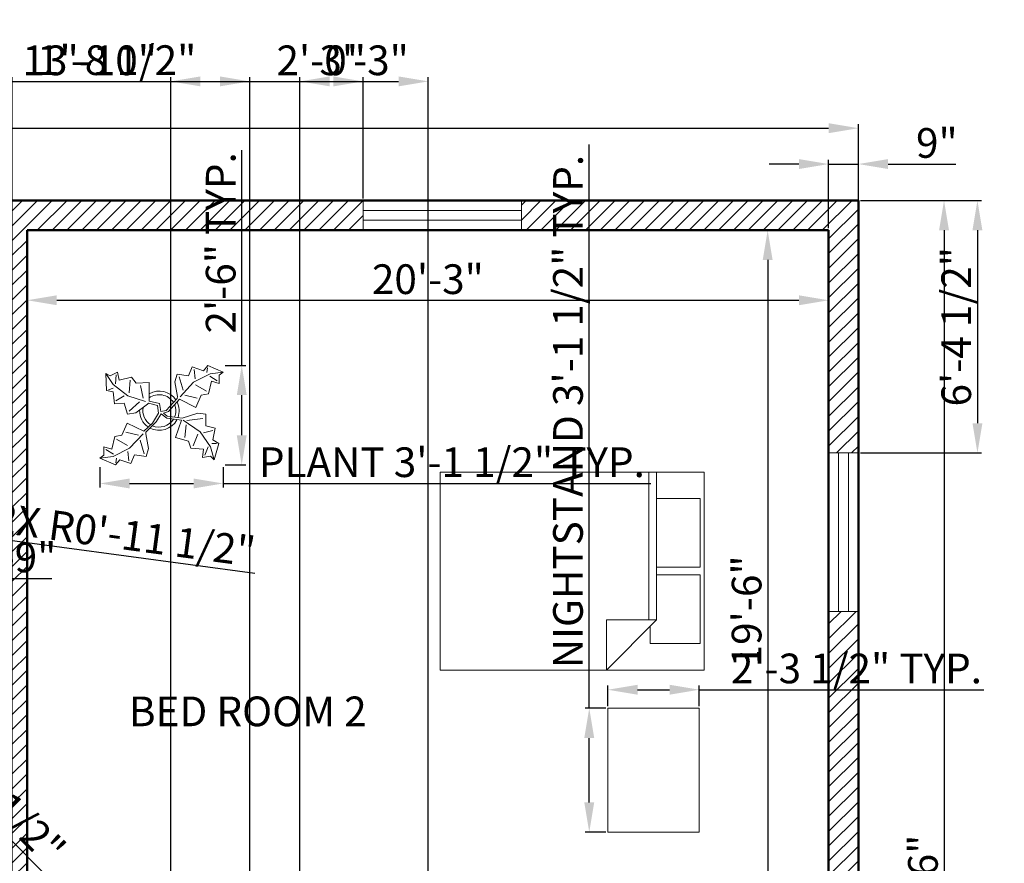
# Model space of a CAD drawing. Units: inches. Extents: x 61993 to 62774, y 55335 to 55871.
# Tile 6 of 6: x 62474 to 62772, y 55615 to 55871. Entities that reach past the tile are written whole.
import ezdxf

# ---------------------------------------------------------------- set-up
doc = ezdxf.new("R2010")
doc.units = ezdxf.units.IN
for name, color, linetype, lineweight in [('A-ANNO-DIMS', 2, 'Continuous', 18), ('A-AREA-IDEN', 7, 'Continuous', 25), ('A-FURN', 9, 'Continuous', 18), ('A-FURN-PLNT', 94, 'Continuous', 13), ('A-GLAZ', 4, 'Continuous', 18), ('A-WALL', 7, 'Continuous', 50)]:
    doc.layers.add(name, color=color, linetype=linetype, lineweight=lineweight)
doc.layers.add('A-WALL-PATT', color=40, linetype='Continuous', lineweight=13, true_color=0xf8d731)
doc.styles.get("Standard").update_dxf_attribs({"font": 'arial.ttf'})
doc.dimstyles.new('ISO-25', dxfattribs={"dimtxt": 9, "dimasz": 9, "dimexe": 1.25, "dimexo": 0.625, "dimtad": 1, "dimdec": 1, "dimrnd": 9, "dimlunit": 3, "dimtxsty": 'Standard', "dimcen": 2.5, "dimadec": 0, "dimazin": 0, "dimtfac": 1, "dimtdec": 1, "dimtmove": 0, "dimatfit": 3, "dimfxl": 1, "dimarcsym": 0})

# ---------------------------------------------------------------- blocks, each defined once
blk = doc.blocks.new('*D7')
at = {"layer": 'A-ANNO-DIMS', "color": 0, "lineweight": -2, "transparency": 16777216}
for p, q in [((62718.57, 55806.96), (62699.45, 55806.96)), ((62700.7, 55797.96), (62700.7, 55584.96)), ((62718.57, 55575.96), (62699.45, 55575.96))]:
    blk.add_line(p, q, dxfattribs=at)
at = {"layer": 'A-ANNO-DIMS', "color": 0, "transparency": 16777216}
for points in [[(62699.2, 55797.96), (62702.2, 55797.96), (62700.7, 55806.96)], [(62699.2, 55584.96), (62702.2, 55584.96), (62700.7, 55575.96)]]:
    blk.add_solid(points, dxfattribs=at)
at = {"layer": 'Defpoints', "color": 0, "transparency": 16777216}
for p in [(62719.19, 55806.96), (62700.7, 55575.96), (62719.19, 55575.96)]:
    blk.add_point(p, dxfattribs=at)
at = {"layer": 'A-ANNO-DIMS', "color": 0, "transparency": 16777216, "insert": (62695.48, 55691.46), "char_height": 9, "attachment_point": 5, "rotation": 90}
blk.add_mtext('19\'-6"', dxfattribs=at)
blk = doc.blocks.new('*D8')
at = {"layer": 'A-ANNO-DIMS', "color": 0, "lineweight": -2, "transparency": 16777216}
for p, q in [((62476.19, 55806.33), (62476.19, 55784.49)), ((62719.19, 55806.33), (62719.19, 55784.49)), ((62485.19, 55785.74), (62710.19, 55785.74))]:
    blk.add_line(p, q, dxfattribs=at)
at = {"layer": 'A-ANNO-DIMS', "color": 0, "transparency": 16777216}
for points in [[(62485.19, 55787.24), (62485.19, 55784.24), (62476.19, 55785.74)], [(62710.19, 55787.24), (62710.19, 55784.24), (62719.19, 55785.74)]]:
    blk.add_solid(points, dxfattribs=at)
at = {"layer": 'Defpoints', "color": 0, "transparency": 16777216}
for p in [(62476.19, 55806.96), (62719.19, 55806.96), (62719.19, 55785.74)]:
    blk.add_point(p, dxfattribs=at)
at = {"layer": 'A-ANNO-DIMS', "color": 0, "transparency": 16777216, "insert": (62597.69, 55790.96), "char_height": 9, "attachment_point": 5}
blk.add_mtext('20\'-3"', dxfattribs=at)
blk = doc.blocks.new('Bed - Queen')
for p, q in [((0, -80.00003), (0, 0)), ((0, 0), (59.99999, 0)), ((59.99999, 0), (59.99999, -80.00003)), ((7.99999, -1.2), (28.79998, -1.2)), ((7.99999, -14.4), (7.99999, -1.2)), ((28.79998, -1.2), (28.79998, -14.4)), ((31.19999, -1.2), (51.99999, -1.2)), ((31.19999, -14.4), (31.19999, -1.2)), ((51.99999, -1.2), (51.99999, -16.4)), ((0, -14.4), (44.8, -14.4)), ((59.99999, -29.6), (44.8, -14.4)), ((44.8, -14.4), (44.8, -29.6)), ((44.8, -16.8), (0, -16.8)), ((51.99999, -16.4), (46.79936, -16.4)), ((44.8, -29.6), (59.99999, -29.6)), ((59.99999, -80.00003), (0, -80.00003))]:
    blk.add_line(p, q)
blk = doc.blocks.new('Plant - Rubber or Philodendron')
for p, q in [((8.8871, 10.7908), (9.9809, 13.4933)), ((9.9809, 13.4933), (13.3837, 12.301)), ((10.5828, 12.6946), (10.8893, 9.7953)), ((13.3837, 12.301), (14.68, 13.9039)), ((14.5816, 13.2037), (14.3848, 11.8033)), ((14.68, 13.9039), (19.3848, 11.8146)), ((-16.2005, 11.4774), (-13.9899, 8.1064)), ((-16.2005, 11.4774), (-14.8639, 10.7964)), ((-16.0159, 6.3329), (-16.2005, 11.4774)), ((-14.8639, 10.7964), (-12.6195, 11.8975)), ((-13.3174, 8.325), (-13.0735, 11.0065)), ((-12.6195, 11.8975), (-12.1909, 9.4345)), ((-12.1909, 9.4345), (-8.3829, 10.3)), ((-8.8369, 9.409), (-9.0894, 5.6095)), ((-8.3829, 10.3), (-7.0549, 8.501)), ((4.6914, 8.8812), (5.3859, 11.2828)), ((5.3859, 11.2828), (8.8871, 10.7908)), ((5.9878, 10.4842), (7.1971, 6.3869)), ((15.3859, 11.3055), (10.3916, 8.7942)), ((15.7909, 9.1065), (14.8995, 5.3044)), ((15.2875, 10.6053), (17.5907, 9.2105)), ((19.3848, 11.8146), (15.3859, 11.3055)), ((18.1925, 8.4119), (15.7909, 9.1065)), ((19.3848, 11.8146), (18.1868, 10.9119)), ((18.1868, 10.9119), (18.1925, 8.4119)), ((-14.0069, 5.8704), (-16.0159, 6.3329)), ((-15.3434, 6.5514), (-13.9984, 6.9884)), ((-13.9899, 8.1064), (-9.5434, 4.7185)), ((-7.0549, 8.501), (-3.0284, 8.6941)), ((-4.8529, 4.012), (-5.7184, 7.82)), ((-3.0284, 8.6941), (-3.0709, 3.1041)), ((4.6914, 8.8812), (5.5014, 4.4831)), ((10.3916, 8.7942), (6.2847, 4.4028)), ((14.2977, 6.1031), (10.9934, 7.9956)), ((-13.5868, 2.2894), (-14.0069, 5.8704)), ((-13.1329, 3.1804), (-10.6614, 4.727)), ((-9.5434, 4.7185), (-4.1917, 2.9888)), ((-3.0709, 3.1041), (0.0797, 2.3163)), ((2.1141, 0.2298), (5.4346, 3.9146)), ((6.1032, 3.6844), (2.8262, -0.031)), ((5.4346, 3.9146), (5.5014, 4.4831)), ((11.1089, 1.1958), (6.1032, 3.6844)), ((7.7005, 4.8881), (11.5025, 3.9967)), ((12.7005, 4.8994), (11.1089, 1.1958)), ((14.8995, 5.3044), (12.7005, 4.8994)), ((-10.6784, 2.491), (-13.5868, 2.2894)), ((-9.5858, -0.8715), (-10.6784, 2.491)), ((-9.1318, 0.0195), (-5.9793, 2.9025)), ((-7.1228, -0.443), (-3.5248, 2.2131)), ((-3.5248, 2.2131), (-3.3011, 2.4355)), ((-3.3011, 2.4355), (-0.5306, 1.7947)), ((-0.5306, 1.7947), (-0.2255, -0.5527)), ((-0.5306, 1.7947), (-0.5306, 1.7947)), ((0.0797, 2.3163), (0.4866, -0.031)), ((0.4866, -0.031), (2.1141, 0.2298)), ((-7.1228, -0.443), (-9.5858, -0.8715)), ((-2.019, -3.6148), (-0.2255, -0.5527)), ((-0.9375, -3.1608), (0.5883, -0.8135)), ((0.5883, -0.8135), (2.2447, -2.0916)), ((2.8262, -0.031), (1.3003, -0.5527)), ((1.3003, -0.5527), (2.4193, -1.4655)), ((2.2447, -2.0916), (6.7108, -2.6626)), ((2.4193, -1.4655), (6.895, -2.1175)), ((4.943, -7.9659), (6.7108, -2.6626)), ((11.6605, -0.5413), (6.895, -2.1175)), ((12.3677, -6.1981), (7.219, -2.6772)), ((8.3544, -2.7453), (13.1973, -2.1704)), ((11.6605, -0.5413), (14.1354, -0.8948)), ((14.1354, -0.8948), (14.1354, -4.4304)), ((-11.3237, -7.2629), (-9.7321, -3.5593)), ((-9.7321, -3.5593), (-4.7264, -6.0479)), ((-2.019, -3.6148), (-4.7264, -6.0479)), ((-4.0579, -6.2781), (-0.9375, -3.1608)), ((8.125, -4.0768), (7.7715, -7.9659)), ((16.2567, -5.8446), (13.4283, -6.5517)), ((14.1354, -4.4304), (16.9638, -5.1375)), ((16.9638, -5.1375), (16.2567, -8.673)), ((-14.4141, -11.4699), (-13.5228, -7.6679)), ((-13.5228, -7.6679), (-11.3237, -7.2629)), ((-12.921, -8.4665), (-9.6166, -10.359)), ((-6.3237, -7.2516), (-10.1257, -6.3602)), ((-9.0148, -11.1577), (-4.9047, -6.8122)), ((-4.611, -12.8477), (-5.8203, -8.7504)), ((-4.1246, -6.8466), (-4.0579, -6.2781)), ((-3.3146, -11.2447), (-4.1246, -6.8466)), ((8.8321, -9.0266), (4.943, -7.9659)), ((10.2463, -10.4408), (11.6605, -6.9053)), ((15.5496, -10.7943), (12.3677, -6.1981)), ((16.2567, -8.673), (18.0245, -9.7337)), ((-16.8157, -10.7754), (-14.4141, -11.4699)), ((-16.8101, -13.2754), (-16.8157, -10.7754)), ((-13.9107, -12.9688), (-16.2139, -11.574)), ((-14.0091, -13.669), (-9.0148, -11.1577)), ((-3.3146, -11.2447), (-4.0092, -13.6463)), ((9.5392, -11.1479), (8.8321, -9.0266)), ((13.4283, -11.5015), (9.5392, -11.1479)), ((13.0748, -13.9763), (13.4283, -11.5015)), ((14.8425, -10.7943), (13.7819, -13.2692)), ((16.6103, -14.6834), (15.5496, -10.7943)), ((17.3174, -9.7337), (15.9032, -9.7337)), ((18.0245, -9.7337), (16.6103, -14.6834)), ((-18.008, -14.1781), (-16.8101, -13.2754)), ((-18.008, -14.1781), (-14.0091, -13.669)), ((-13.3032, -16.2674), (-18.008, -14.1781)), ((-12.0069, -14.6645), (-13.3032, -16.2674)), ((-13.2048, -15.5672), (-13.008, -14.1668)), ((-8.6042, -15.8568), (-12.0069, -14.6645)), ((-9.206, -15.0581), (-9.5126, -12.1588)), ((-7.5103, -13.1543), (-8.6042, -15.8568)), ((-4.0092, -13.6463), (-7.5103, -13.1543)), ((15.5496, -13.6228), (13.0748, -13.9763)), ((16.6103, -14.6834), (15.5496, -13.6228))]:
    blk.add_line(p, q)
for centre, radius, start, end in [((0, 0), 6.1275, 34.37569, 120.1028), ((-0.0601, -0.2075), 5.2461, 33.82192, 124.9414), ((0.0308, 0.1664), 6, 178.6147, 235.1169), ((0.0308, 0.1664), 5, 168.1647, 238.6725), ((-0.2664, 0.1682), 5.2775, 338.4094, 20.03007), ((-0.098, 0.1364), 6.1288, 341.2017, 26.09184), ((-0.0234, 0.3825), 6.1492, 242.5812, 331.2714), ((-0.1102, 0.4886), 5.2883, 247.3711, 327.472)]:
    blk.add_arc(centre, radius, start, end)
blk = doc.blocks.new('*D24')
at = {"layer": 'A-ANNO-DIMS', "color": 0, "lineweight": -2, "transparency": 16777216}
for p, q in [((62068.19, 55816.58), (62068.19, 55839.13)), ((62728.19, 55816.58), (62728.19, 55839.13)), ((62077.19, 55837.88), (62719.19, 55837.88))]:
    blk.add_line(p, q, dxfattribs=at)
at = {"layer": 'A-ANNO-DIMS', "color": 0, "transparency": 16777216}
for points in [[(62077.19, 55839.38), (62077.19, 55836.38), (62068.19, 55837.88)], [(62719.19, 55839.38), (62719.19, 55836.38), (62728.19, 55837.88)]]:
    blk.add_solid(points, dxfattribs=at)
at = {"layer": 'Defpoints', "color": 0, "transparency": 16777216}
for p in [(62728.19, 55837.88), (62068.19, 55815.96), (62728.19, 55815.96)]:
    blk.add_point(p, dxfattribs=at)
at = {"layer": 'A-ANNO-DIMS', "color": 0, "transparency": 16777216, "insert": (62398.19, 55843.1), "char_height": 9, "attachment_point": 5}
blk.add_mtext('54\'-9"', dxfattribs=at)
blk = doc.blocks.new('*D25')
at = {"layer": 'A-ANNO-DIMS', "color": 0, "lineweight": -2, "transparency": 16777216}
for p, q in [((62728.82, 55815.96), (62755.41, 55815.96)), ((62754.16, 55806.96), (62754.16, 55406.74)), ((62728.82, 55397.74), (62755.41, 55397.74))]:
    blk.add_line(p, q, dxfattribs=at)
at = {"layer": 'A-ANNO-DIMS', "color": 0, "transparency": 16777216}
for points in [[(62752.66, 55806.96), (62755.66, 55806.96), (62754.16, 55815.96)], [(62752.66, 55406.74), (62755.66, 55406.74), (62754.16, 55397.74)]]:
    blk.add_solid(points, dxfattribs=at)
at = {"layer": 'Defpoints', "color": 0, "transparency": 16777216}
for p in [(62728.19, 55815.96), (62728.19, 55397.74), (62754.16, 55397.74)]:
    blk.add_point(p, dxfattribs=at)
at = {"layer": 'A-ANNO-DIMS', "color": 0, "transparency": 16777216, "insert": (62748.93, 55606.85), "char_height": 9, "attachment_point": 5, "rotation": 90}
blk.add_mtext('34\'-6"', dxfattribs=at)
blk = doc.blocks.new('*D26')
at = {"layer": 'A-ANNO-DIMS', "color": 0, "lineweight": -2, "transparency": 16777216}
for p, q in [((62719.19, 55807.58), (62719.19, 55828.27)), ((62728.19, 55807.58), (62728.19, 55828.27)), ((62710.19, 55827.02), (62701.19, 55827.02)), ((62719.19, 55827.02), (62728.19, 55827.02)), ((62737.19, 55827.02), (62757.79, 55827.02))]:
    blk.add_line(p, q, dxfattribs=at)
at = {"layer": 'A-ANNO-DIMS', "color": 0, "transparency": 16777216}
for points in [[(62710.19, 55828.52), (62710.19, 55825.52), (62719.19, 55827.02)], [(62737.19, 55828.52), (62737.19, 55825.52), (62728.19, 55827.02)]]:
    blk.add_solid(points, dxfattribs=at)
at = {"layer": 'Defpoints', "color": 0, "transparency": 16777216}
for p in [(62728.19, 55827.02), (62719.19, 55806.96), (62728.19, 55806.96)]:
    blk.add_point(p, dxfattribs=at)
at = {"layer": 'A-ANNO-DIMS', "color": 0, "transparency": 16777216, "insert": (62751.99, 55832.24), "char_height": 9, "attachment_point": 5}
blk.add_mtext('9"', dxfattribs=at)
blk = doc.blocks.new('WIN-48IN')
for p, q in [((0, 9), (0, 0)), ((48, 9), (48, 0)), ((48, 6), (0, 6)), ((48, 3), (0, 3))]:
    blk.add_line(p, q)
blk = doc.blocks.new('TABLE-BEDSIDE')
blk.add_lwpolyline([(0, 37.52), (27.74, 37.52), (27.74, 0), (0, 0)], close=True)
blk = doc.blocks.new('*D36')
at = {"layer": 'A-ANNO-DIMS', "color": 0, "lineweight": -2, "transparency": 16777216}
for p, q in [((62498.26, 55735.2), (62498.26, 55728.97)), ((62535.65, 55735.2), (62535.65, 55728.97)), ((62507.26, 55730.22), (62526.65, 55730.22)), ((62535.65, 55730.22), (62665.3, 55730.22))]:
    blk.add_line(p, q, dxfattribs=at)
at = {"layer": 'A-ANNO-DIMS', "color": 0, "transparency": 16777216}
for points in [[(62507.26, 55731.72), (62507.26, 55728.72), (62498.26, 55730.22)], [(62526.65, 55731.72), (62526.65, 55728.72), (62535.65, 55730.22)]]:
    blk.add_solid(points, dxfattribs=at)
at = {"layer": 'Defpoints', "color": 0, "transparency": 16777216}
for p in [(62498.26, 55735.83), (62535.65, 55735.83), (62535.65, 55730.22)]:
    blk.add_point(p, dxfattribs=at)
at = {"layer": 'A-ANNO-DIMS', "color": 0, "transparency": 16777216, "insert": (62604.97, 55735.5), "char_height": 9, "attachment_point": 5}
blk.add_mtext('PLANT 3\'-1 1/2" TYP.', dxfattribs=at)
blk = doc.blocks.new('*D37')
at = {"layer": 'A-ANNO-DIMS', "color": 0, "lineweight": -2, "transparency": 16777216}
for p, q in [((62541.26, 55766), (62541.26, 55831.26)), ((62536.27, 55766), (62542.51, 55766)), ((62541.26, 55744.83), (62541.26, 55757)), ((62536.27, 55735.83), (62542.51, 55735.83))]:
    blk.add_line(p, q, dxfattribs=at)
at = {"layer": 'A-ANNO-DIMS', "color": 0, "transparency": 16777216}
for points in [[(62539.76, 55757), (62542.76, 55757), (62541.26, 55766)], [(62539.76, 55744.83), (62542.76, 55744.83), (62541.26, 55735.83)]]:
    blk.add_solid(points, dxfattribs=at)
at = {"layer": 'Defpoints', "color": 0, "transparency": 16777216}
for p in [(62535.65, 55766), (62541.26, 55766), (62535.65, 55735.83)]:
    blk.add_point(p, dxfattribs=at)
at = {"layer": 'A-ANNO-DIMS', "color": 0, "transparency": 16777216, "insert": (62536.04, 55803.13), "char_height": 9, "attachment_point": 5, "rotation": 90}
blk.add_mtext('2\'-6" TYP.', dxfattribs=at)
blk = doc.blocks.new('*D40')
at = {"layer": 'A-ANNO-DIMS', "color": 0, "lineweight": -2, "transparency": 16777216}
for p, q in [((62646.61, 55662.09), (62646.61, 55832.95)), ((62651.61, 55662.09), (62645.36, 55662.09)), ((62646.61, 55633.57), (62646.61, 55653.09)), ((62651.61, 55624.57), (62645.36, 55624.57))]:
    blk.add_line(p, q, dxfattribs=at)
at = {"layer": 'A-ANNO-DIMS', "color": 0, "transparency": 16777216}
for points in [[(62645.11, 55653.09), (62648.11, 55653.09), (62646.61, 55662.09)], [(62645.11, 55633.57), (62648.11, 55633.57), (62646.61, 55624.57)]]:
    blk.add_solid(points, dxfattribs=at)
at = {"layer": 'Defpoints', "color": 0, "transparency": 16777216}
for p in [(62646.61, 55662.09), (62652.24, 55662.09), (62652.24, 55624.57)]:
    blk.add_point(p, dxfattribs=at)
at = {"layer": 'A-ANNO-DIMS', "color": 0, "transparency": 16777216, "insert": (62641.33, 55752.02), "char_height": 9, "attachment_point": 5, "rotation": 90}
blk.add_mtext('NIGHTSTAND 3\'-1 1/2" TYP.', dxfattribs=at)
blk = doc.blocks.new('*D41')
at = {"layer": 'A-ANNO-DIMS', "color": 0, "lineweight": -2, "transparency": 16777216}
for p, q in [((62652.24, 55662.71), (62652.24, 55668.97)), ((62679.98, 55662.71), (62679.98, 55668.97)), ((62661.24, 55667.72), (62670.98, 55667.72)), ((62679.98, 55667.72), (62766.22, 55667.72))]:
    blk.add_line(p, q, dxfattribs=at)
at = {"layer": 'A-ANNO-DIMS', "color": 0, "transparency": 16777216}
for points in [[(62661.24, 55669.22), (62661.24, 55666.22), (62652.24, 55667.72)], [(62670.98, 55669.22), (62670.98, 55666.22), (62679.98, 55667.72)]]:
    blk.add_solid(points, dxfattribs=at)
at = {"layer": 'Defpoints', "color": 0, "transparency": 16777216}
for p in [(62679.98, 55667.72), (62652.24, 55662.09), (62679.98, 55662.09)]:
    blk.add_point(p, dxfattribs=at)
at = {"layer": 'A-ANNO-DIMS', "color": 0, "transparency": 16777216, "insert": (62727.6, 55673), "char_height": 9, "attachment_point": 5}
blk.add_mtext('2\'-3 1/2" TYP.', dxfattribs=at)
blk = doc.blocks.new('*D45')
at = {"layer": 'A-ANNO-DIMS', "color": 0, "lineweight": -2, "transparency": 16777216}
for p, q in [((62429.34, 55705.79), (62429.34, 55700.2)), ((62450.34, 55705.79), (62450.34, 55700.2)), ((62438.34, 55701.45), (62441.34, 55701.45)), ((62450.34, 55701.45), (62483.66, 55701.45))]:
    blk.add_line(p, q, dxfattribs=at)
at = {"layer": 'A-ANNO-DIMS', "color": 0, "transparency": 16777216}
for points in [[(62438.34, 55702.95), (62438.34, 55699.95), (62429.34, 55701.45)], [(62441.34, 55702.95), (62441.34, 55699.95), (62450.34, 55701.45)]]:
    blk.add_solid(points, dxfattribs=at)
at = {"layer": 'Defpoints', "color": 0, "transparency": 16777216}
for p in [(62429.34, 55706.41), (62450.34, 55706.41), (62450.34, 55701.45)]:
    blk.add_point(p, dxfattribs=at)
at = {"layer": 'A-ANNO-DIMS', "color": 0, "transparency": 16777216, "insert": (62471.5, 55706.67), "char_height": 9, "attachment_point": 5}
blk.add_mtext('1\'-9"', dxfattribs=at)
blk = doc.blocks.new('*D66')
at = {"layer": 'A-ANNO-DIMS', "color": 0, "lineweight": -2, "transparency": 16777216}
for p, q in [((62412.31, 55816.58), (62412.31, 55853.31)), ((62421.31, 55852.06), (62569.07, 55852.06)), ((62578.07, 55816.58), (62578.07, 55853.31))]:
    blk.add_line(p, q, dxfattribs=at)
at = {"layer": 'A-ANNO-DIMS', "color": 0, "transparency": 16777216}
for points in [[(62421.31, 55853.56), (62421.31, 55850.56), (62412.31, 55852.06)], [(62569.07, 55853.56), (62569.07, 55850.56), (62578.07, 55852.06)]]:
    blk.add_solid(points, dxfattribs=at)
at = {"layer": 'Defpoints', "color": 0, "transparency": 16777216}
for p in [(62578.07, 55852.06), (62412.31, 55815.96), (62578.07, 55815.96)]:
    blk.add_point(p, dxfattribs=at)
at = {"layer": 'A-ANNO-DIMS', "color": 0, "transparency": 16777216, "insert": (62495.19, 55857.28), "char_height": 9, "attachment_point": 5}
blk.add_mtext('13\'-10"', dxfattribs=at)
blk = doc.blocks.new('*D69')
at = {"layer": 'A-ANNO-DIMS', "color": 0, "lineweight": -2, "transparency": 16777216}
for p, q in [((62728.82, 55815.96), (62765.54, 55815.96)), ((62764.29, 55806.96), (62764.29, 55748.46)), ((62728.82, 55739.46), (62765.54, 55739.46))]:
    blk.add_line(p, q, dxfattribs=at)
at = {"layer": 'A-ANNO-DIMS', "color": 0, "transparency": 16777216}
for points in [[(62762.79, 55806.96), (62765.79, 55806.96), (62764.29, 55815.96)], [(62762.79, 55748.46), (62765.79, 55748.46), (62764.29, 55739.46)]]:
    blk.add_solid(points, dxfattribs=at)
at = {"layer": 'Defpoints', "color": 0, "transparency": 16777216}
for p in [(62728.19, 55815.96), (62728.19, 55739.46), (62764.29, 55739.46)]:
    blk.add_point(p, dxfattribs=at)
at = {"layer": 'A-ANNO-DIMS', "color": 0, "transparency": 16777216, "insert": (62759.02, 55777.71), "char_height": 9, "attachment_point": 5, "rotation": 90}
blk.add_mtext('6\'-4 1/2"', dxfattribs=at)
blk = doc.blocks.new('*D72')
at = {"layer": 'A-ANNO-DIMS', "color": 0, "lineweight": -2, "transparency": 16777216}
for p, q in [((62451.32, 55576.58), (62451.32, 55853.31)), ((62460.32, 55852.06), (62462.69, 55852.06)), ((62471.69, 55576.58), (62471.69, 55853.31)), ((62471.69, 55852.06), (62525.99, 55852.06))]:
    blk.add_line(p, q, dxfattribs=at)
at = {"layer": 'A-ANNO-DIMS', "color": 0, "transparency": 16777216}
for points in [[(62460.32, 55853.56), (62460.32, 55850.56), (62451.32, 55852.06)], [(62462.69, 55853.56), (62462.69, 55850.56), (62471.69, 55852.06)]]:
    blk.add_solid(points, dxfattribs=at)
at = {"layer": 'Defpoints', "color": 0, "transparency": 16777216}
for p in [(62471.69, 55852.06), (62451.32, 55575.96), (62471.69, 55575.96)]:
    blk.add_point(p, dxfattribs=at)
at = {"layer": 'A-ANNO-DIMS', "color": 0, "transparency": 16777216, "insert": (62503.34, 55857.33), "char_height": 9, "attachment_point": 5}
blk.add_mtext('1\'-8 1/2"', dxfattribs=at)
blk = doc.blocks.new('*D73')
at = {"layer": 'A-ANNO-DIMS', "color": 0, "lineweight": -2, "transparency": 16777216}
for p, q in [((62519.74, 55576.58), (62519.74, 55853.31)), ((62528.74, 55852.06), (62534.69, 55852.06)), ((62543.69, 55572.08), (62543.69, 55853.31)), ((62543.69, 55852.06), (62578.02, 55852.06))]:
    blk.add_line(p, q, dxfattribs=at)
at = {"layer": 'A-ANNO-DIMS', "color": 0, "transparency": 16777216}
for points in [[(62528.74, 55853.56), (62528.74, 55850.56), (62519.74, 55852.06)], [(62534.69, 55853.56), (62534.69, 55850.56), (62543.69, 55852.06)]]:
    blk.add_solid(points, dxfattribs=at)
at = {"layer": 'Defpoints', "color": 0, "transparency": 16777216}
for p in [(62543.69, 55852.06), (62519.74, 55575.96), (62543.69, 55571.46)]:
    blk.add_point(p, dxfattribs=at)
at = {"layer": 'A-ANNO-DIMS', "color": 0, "transparency": 16777216, "insert": (62565.36, 55857.28), "char_height": 9, "attachment_point": 5}
blk.add_mtext('2\'-0"', dxfattribs=at)
blk = doc.blocks.new('*D79')
at = {"layer": 'A-ANNO-DIMS', "color": 0, "lineweight": -2, "transparency": 16777216}
for p, q in [((62558.91, 55496.8), (62558.91, 55853.31)), ((62567.91, 55852.06), (62588.8, 55852.06)), ((62597.8, 55496.8), (62597.8, 55853.31))]:
    blk.add_line(p, q, dxfattribs=at)
at = {"layer": 'A-ANNO-DIMS', "color": 0, "transparency": 16777216}
for points in [[(62567.91, 55853.56), (62567.91, 55850.56), (62558.91, 55852.06)], [(62588.8, 55853.56), (62588.8, 55850.56), (62597.8, 55852.06)]]:
    blk.add_solid(points, dxfattribs=at)
at = {"layer": 'Defpoints', "color": 0, "transparency": 16777216}
for p in [(62597.8, 55852.06), (62558.91, 55496.17), (62597.8, 55496.17)]:
    blk.add_point(p, dxfattribs=at)
at = {"layer": 'A-ANNO-DIMS', "color": 0, "transparency": 16777216, "insert": (62578.36, 55857.28), "char_height": 9, "attachment_point": 5}
blk.add_mtext('3\'-3"', dxfattribs=at)
blk = doc.blocks.new('*D87')
at = {"layer": 'A-ANNO-DIMS', "color": 0, "lineweight": -2, "transparency": 16777216}
for p, q in [((62424.07, 55669.37), (62487.77, 55605.68)), ((62519.24, 55574.21), (62494.13, 55599.31))]:
    blk.add_line(p, q, dxfattribs=at)
at = {"layer": 'A-ANNO-DIMS', "color": 0, "transparency": 16777216}
blk.add_solid([(62488.83, 55606.74), (62486.71, 55604.61), (62494.13, 55599.31)], dxfattribs=at)
at = {"layer": 'Defpoints', "color": 0, "transparency": 16777216}
for p in [(62494.13, 55599.31), (62519.24, 55574.21)]:
    blk.add_point(p, dxfattribs=at)
at = {"layer": 'A-ANNO-DIMS', "color": 0, "transparency": 16777216, "insert": (62456.47, 55644.44), "char_height": 9, "attachment_point": 5, "rotation": 315}
blk.add_mtext('3X R2\'-11 1/2"', dxfattribs=at)
blk = doc.blocks.new('*D90')
at = {"layer": 'A-ANNO-DIMS', "color": 0, "lineweight": -2, "transparency": 16777216}
for p, q in [((62435.64, 55717.64), (62446.86, 55716.13)), ((62545.22, 55702.9), (62455.78, 55714.93))]:
    blk.add_line(p, q, dxfattribs=at)
at = {"layer": 'A-ANNO-DIMS', "color": 0, "transparency": 16777216}
blk.add_solid([(62455.98, 55716.42), (62455.58, 55713.44), (62446.86, 55716.13)], dxfattribs=at)
at = {"layer": 'Defpoints', "color": 0, "transparency": 16777216}
for p in [(62435.64, 55717.64), (62446.86, 55716.13)]:
    blk.add_point(p, dxfattribs=at)
at = {"layer": 'A-ANNO-DIMS', "color": 0, "transparency": 16777216, "insert": (62505.67, 55713.55), "char_height": 9, "attachment_point": 5, "rotation": 352.3402}
blk.add_mtext('2X R0\'-11 1/2"', dxfattribs=at)

msp = doc.modelspace()

# ---------------------------------------------------------------- hatches: boundary and pattern name
at = {"layer": 'A-WALL-PATT'}
h = msp.add_hatch(dxfattribs=at)
h.set_pattern_fill('ANSI31', color=256)
h.paths.add_polyline_path([(62077.19, 55665.16), (62068.19, 55665.16), (62068.19, 55518.96), (62077.19, 55518.96), (62077.19, 55571.46), (62234.23, 55571.46), (62234.23, 55573.71, -0.007042), (62234.23, 55574.71), (62234.23, 55575.96), (62077.19, 55575.96)])
h.paths.add_polyline_path([(62077.19, 55806.96), (62138.51, 55806.96), (62138.51, 55815.96), (62068.19, 55815.96), (62068.19, 55713.16), (62077.19, 55713.16)])
h.paths.add_polyline_path([(62364.31, 55815.96), (62186.51, 55815.96), (62186.51, 55806.96), (62308.19, 55806.96), (62308.19, 55575.96), (62270.23, 55575.96), (62270.23, 55571.46), (62415.32, 55571.46), (62415.32, 55573.71, -0.007042), (62415.32, 55574.71), (62415.32, 55575.96), (62312.69, 55575.96), (62312.69, 55739.46), (62471.69, 55739.46), (62471.69, 55575.96), (62451.32, 55575.96), (62451.32, 55571.46), (62483.74, 55571.46), (62483.74, 55573.71, -0.007042), (62483.74, 55574.71), (62483.74, 55575.96), (62476.19, 55575.96), (62476.19, 55806.96), (62578.07, 55806.96), (62578.07, 55815.96), (62412.31, 55815.96), (62412.31, 55806.96), (62471.69, 55806.96), (62471.69, 55743.96), (62312.69, 55743.96), (62312.69, 55806.96), (62364.31, 55806.96)])
h.paths.add_polyline_path([(62728.19, 55815.96), (62626.07, 55815.96), (62626.07, 55806.96), (62719.19, 55806.96), (62719.19, 55739.46), (62728.19, 55739.46)])
h.paths.add_polyline_path([(62728.19, 55691.46), (62719.19, 55691.46), (62719.19, 55575.96), (62519.74, 55575.96), (62519.74, 55571.46), (62543.69, 55571.46), (62543.69, 55568.46), (62548.19, 55568.46), (62548.19, 55571.46), (62719.19, 55571.46), (62719.19, 55517.72), (62728.19, 55517.72)])
h.paths.add_polyline_path([(62599.31, 55404.96), (62548.19, 55404.96), (62548.19, 55532.46), (62546.94, 55532.46, -0.007042), (62545.94, 55532.46), (62543.69, 55532.46), (62543.69, 55404.96), (62444.22, 55404.96), (62444.22, 55395.96), (62599.31, 55395.96)])
h.paths.add_polyline_path([(62728.19, 55469.72), (62719.19, 55469.72), (62719.19, 55404.96), (62647.31, 55404.96), (62647.31, 55395.96), (62728.19, 55395.96)])
h.paths.add_polyline_path([(62396.22, 55404.96), (62309.17, 55404.96), (62309.17, 55395.96), (62396.22, 55395.96)])
h.paths.add_polyline_path([(62213.17, 55404.96), (62077.19, 55404.96), (62077.19, 55470.96), (62068.19, 55470.96), (62068.19, 55395.96), (62213.17, 55395.96)])

# ---------------------------------------------------------------- linework, layer by layer
at = {"layer": 'A-WALL'}
for p, q in [((62728.19, 55815.96), (62068.19, 55815.96)), ((62728.19, 55395.96), (62728.19, 55815.96)), ((62719.19, 55806.96), (62476.19, 55806.96)), ((62476.19, 55806.96), (62476.19, 55575.96)), ((62719.19, 55575.96), (62719.19, 55806.96))]:
    msp.add_line(p, q, dxfattribs=at)

# ---------------------------------------------------------------- block references
at = {"layer": 'A-FURN', "rotation": 270}
msp.add_blockref('Bed - Queen', (62681.44, 55733.69), dxfattribs=at)
at = {"layer": 'A-FURN'}
msp.add_blockref('TABLE-BEDSIDE', (62652.24, 55624.57), dxfattribs=at)
at = {"layer": 'A-FURN-PLNT'}
msp.add_blockref('Plant - Rubber or Philodendron', (62516.26, 55752.09), dxfattribs=at)
at = {"layer": 'A-GLAZ'}
msp.add_blockref('WIN-48IN', (62578.07, 55806.96), dxfattribs=at)
at = {"layer": 'A-GLAZ', "rotation": 269.9999999999937}
msp.add_blockref('WIN-48IN', (62719.19, 55739.46), dxfattribs=at)

# ---------------------------------------------------------------- texts
at = {"layer": 'A-AREA-IDEN', "insert": (62507.08, 55665.66), "char_height": 9, "attachment_point": 1}
msp.add_mtext_dynamic_manual_height_columns('BED ROOM 2', width=116.6414, gutter_width=12.5, heights=[0], dxfattribs=at)

# ---------------------------------------------------------------- dimensions: what is measured, and where the dimension line sits
at = {"layer": 'A-ANNO-DIMS'}
for base, p1, p2, override, picture, middle in [((62471.69, 55852.06), (62451.32, 55575.96), (62471.69, 55575.96), {"dimdec": 1, "dimlfac": 1, "dimrnd": 0, "dimzin": 1, "dimdsep": 46, "dimlunit": 4, "dimfrac": 2}, '*D72', (62503.34, 55857.33)), ((62578.07, 55852.06), (62412.31, 55815.96), (62578.07, 55815.96), {"dimdec": 1, "dimlfac": 1, "dimrnd": 0, "dimzin": 1, "dimdsep": 46, "dimlunit": 4, "dimfrac": 2}, '*D66', (62495.19, 55857.28)), ((62543.6945, 55852.0565), (62519.7385, 55575.9565), (62543.6945, 55571.4565), {"dimdec": 1, "dimlfac": 1, "dimrnd": 0, "dimzin": 1, "dimdsep": 46, "dimlunit": 4, "dimfrac": 2}, '*D73', (62565.3584, 55857.2767)), ((62597.8, 55852.06), (62558.91, 55496.17), (62597.8, 55496.17), {"dimdec": 1, "dimlfac": 1, "dimrnd": 0, "dimzin": 1, "dimdsep": 46, "dimlunit": 4, "dimfrac": 2}, '*D79', (62578.36, 55857.28)), ((62728.19, 55837.88), (62068.19, 55815.96), (62728.19, 55815.96), {"dimclrd": 0, "dimclre": 0, "dimclrt": 0}, '*D24', (62398.19, 55843.1)), ((62728.19, 55827.02), (62719.19, 55806.96), (62728.19, 55806.96), {"dimclrd": 0, "dimclre": 0, "dimclrt": 0}, '*D26', (62751.99, 55832.24)), ((62719.19, 55785.74), (62476.19, 55806.96), (62719.19, 55806.96), {"dimclrd": 0, "dimclre": 0, "dimclrt": 0}, '*D8', (62597.69, 55790.96)), ((62450.34, 55701.45), (62429.34, 55706.41), (62450.34, 55706.41), {"dimdec": 1, "dimlfac": 1, "dimrnd": 0, "dimzin": 1, "dimdsep": 46, "dimlunit": 4, "dimfrac": 2}, '*D45', (62471.5, 55706.67))]:
    dim = msp.add_linear_dim(base=base, p1=p1, p2=p2, dimstyle='ISO-25', override=override, dxfattribs=at)
    dim.commit()
    dim.dimension.update_dxf_attribs({"geometry": picture, "text_midpoint": middle})
for base, p1, p2, text, picture, middle in [((62541.26, 55766), (62535.65, 55735.83), (62535.65, 55766), '<> TYP.', '*D37', (62536.04, 55803.13)), ((62646.61, 55662.09), (62652.24, 55624.57), (62652.24, 55662.09), 'NIGHTSTAND <> TYP.', '*D40', (62641.33, 55752.02))]:
    dim = msp.add_linear_dim(base=base, p1=p1, p2=p2, angle=90, text=text, dimstyle='ISO-25', override={"dimdec": 1, "dimlfac": 1, "dimrnd": 0, "dimzin": 1, "dimdsep": 46, "dimlunit": 4, "dimfrac": 2}, dxfattribs=at)
    dim.commit()
    dim.dimension.update_dxf_attribs({"geometry": picture, "text_midpoint": middle})
for base, p1, p2, override, picture, middle in [((62754.16, 55397.74), (62728.19, 55815.96), (62728.19, 55397.74), {"dimclrd": 0, "dimclre": 0, "dimclrt": 0}, '*D25', (62748.93, 55606.85)), ((62764.29, 55739.46), (62728.19, 55815.96), (62728.19, 55739.46), {"dimdec": 1, "dimlfac": 1, "dimrnd": 0, "dimzin": 1, "dimdsep": 46, "dimlunit": 4, "dimfrac": 2}, '*D69', (62759.02, 55777.71)), ((62700.7, 55575.96), (62719.19, 55806.96), (62719.19, 55575.96), {"dimclrd": 0, "dimclre": 0, "dimclrt": 0}, '*D7', (62695.48, 55691.46))]:
    dim = msp.add_linear_dim(base=base, p1=p1, p2=p2, angle=90, dimstyle='ISO-25', override=override, dxfattribs=at)
    dim.commit()
    dim.dimension.update_dxf_attribs({"geometry": picture, "text_midpoint": middle})
for base, p1, p2, text, picture, middle in [((62535.65, 55730.22), (62498.26, 55735.83), (62535.65, 55735.83), 'PLANT <> TYP.', '*D36', (62604.97, 55735.5)), ((62679.98, 55667.72), (62652.24, 55662.09), (62679.98, 55662.09), '<> TYP.', '*D41', (62727.6, 55673))]:
    dim = msp.add_linear_dim(base=base, p1=p1, p2=p2, text=text, dimstyle='ISO-25', override={"dimdec": 1, "dimlfac": 1, "dimrnd": 0, "dimzin": 1, "dimdsep": 46, "dimlunit": 4, "dimfrac": 2}, dxfattribs=at)
    dim.commit()
    dim.dimension.update_dxf_attribs({"geometry": picture, "text_midpoint": middle})
for center, mpoint, text, picture, middle in [((62435.64, 55717.64), (62446.86, 55716.13), '2X <>', '*D90', (62505.67, 55713.55)), ((62519.24, 55574.21), (62494.13, 55599.31), '3X <>', '*D87', (62456.47, 55644.44))]:
    dim = msp.add_radius_dim(center=center, mpoint=mpoint, text=text, dimstyle='ISO-25', override={"dimdec": 1, "dimlfac": 1, "dimrnd": 0, "dimzin": 1, "dimdsep": 46, "dimlunit": 4, "dimfrac": 2}, dxfattribs=at)
    dim.commit()
    dim.dimension.update_dxf_attribs({"geometry": picture, "text_midpoint": middle})

doc.saveas('drawing.dxf')
